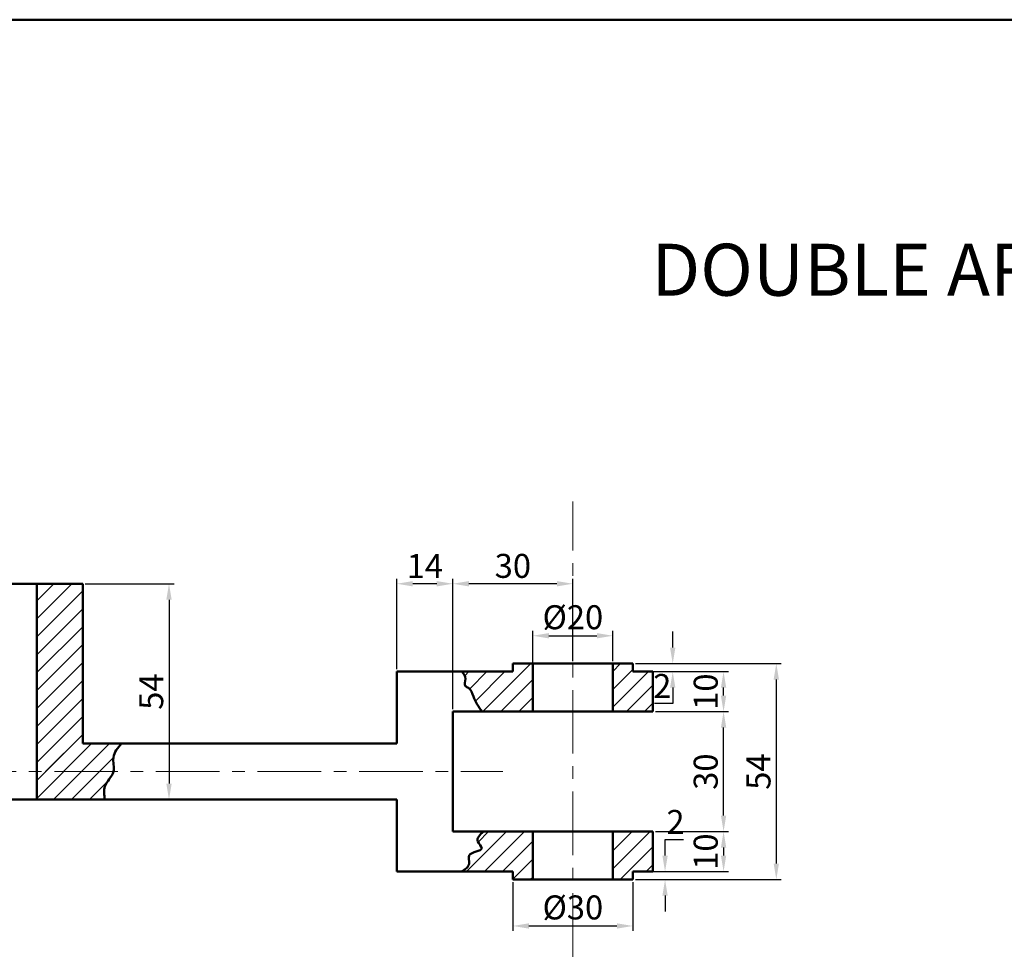
# Model space of a CAD drawing. Units: millimetres. Extents: x -1099 to -222, y 37 to 495.
# Tile 2 of 3: x -920 to -674, y 263 to 495. Entities that reach past the tile are written whole.
import ezdxf

# ---------------------------------------------------------------- set-up
doc = ezdxf.new("R2010")
doc.units = ezdxf.units.MM
doc.header["$LTSCALE"] = 0.5
doc.linetypes.add('CENTER', pattern=[50.800000000000004, 31.75, -6.349999999999999, 6.349999999999999, -6.349999999999999])
for name, color, linetype, lineweight in [('M-CNTR', 1, 'CENTER', 18), ('M-DIMS', 2, 'Continuous', 25), ('M-HATC', 8, 'Continuous', 18), ('M-OUTL', 7, 'Continuous', 50), ('M-TEXT', 7, 'Continuous', 25), ('M-TTLB', 7, 'Continuous', 50)]:
    doc.layers.add(name, color=color, linetype=linetype, lineweight=lineweight)
doc.styles.get("Standard").update_dxf_attribs({"font": 'arial.ttf'})
doc.dimstyles.new('ISO-25', dxfattribs={"dimtxt": 6, "dimasz": 4, "dimexe": 1.25, "dimexo": 0.625, "dimtad": 1, "dimtoh": 1, "dimtxsty": 'Standard', "dimcen": 2.5, "dimadec": 0, "dimazin": 0, "dimtfac": 1, "dimtofl": 0, "dimtmove": 0, "dimatfit": 3, "dimfxl": 1, "dimarcsym": 0})
pattern_1 = [(45, (-1406.913769851486, -374.9261606673909), (-2.245064030267288, 2.245064030267288), [])]

# ---------------------------------------------------------------- blocks, each defined once
blk = doc.blocks.new('*D8')
at = {"layer": 'Defpoints', "color": 0, "transparency": 16777216}
for p in [(-796.41964155178, 280.3451799427145), (-766.41964155178, 280.3451799427145), (-766.41964155178, 268.7543255228883)]:
    blk.add_point(p, dxfattribs=at)
at = {"layer": 'M-DIMS', "color": 0, "lineweight": -2, "transparency": 16777216}
for p, q in [((-796.41964155178, 279.7201799427145), (-796.41964155178, 267.5043255228883)), ((-766.41964155178, 279.7201799427145), (-766.41964155178, 267.5043255228883)), ((-792.41964155178, 268.7543255228883), (-770.41964155178, 268.7543255228883))]:
    blk.add_line(p, q, dxfattribs=at)
at = {"layer": 'M-DIMS', "color": 0, "transparency": 16777216}
for points in [[(-792.41964155178, 269.4209921895549), (-792.41964155178, 268.0876588562216), (-796.41964155178, 268.7543255228883)], [(-770.41964155178, 269.4209921895549), (-770.41964155178, 268.0876588562216), (-766.41964155178, 268.7543255228883)]]:
    blk.add_solid(points, dxfattribs=at)
at = {"layer": 'M-DIMS', "color": 0, "transparency": 16777216, "insert": (-781.41964155178, 272.6105669962853), "char_height": 6, "attachment_point": 5}
blk.add_mtext('%%C30', dxfattribs=at)
blk = doc.blocks.new('*D9')
at = {"layer": 'Defpoints', "color": 0, "transparency": 16777216}
for p in [(-761.4196415517803, 292.3451799427147), (-766.4196415517803, 282.3451799427146), (-743.7539602163725, 282.3451799427146)]:
    blk.add_point(p, dxfattribs=at)
at = {"layer": 'M-DIMS', "color": 0, "lineweight": -2, "transparency": 16777216}
for p, q in [((-760.7946415517802, 292.3451799427147), (-742.5039602163725, 292.3451799427147)), ((-743.7539602163725, 288.3451799427147), (-743.7539602163725, 286.3451799427146)), ((-765.7946415517804, 282.3451799427146), (-742.5039602163725, 282.3451799427146))]:
    blk.add_line(p, q, dxfattribs=at)
at = {"layer": 'M-DIMS', "color": 0, "transparency": 16777216}
for points in [[(-744.4206268830392, 288.3451799427147), (-743.0872935497059, 288.3451799427147), (-743.7539602163725, 292.3451799427147)], [(-744.4206268830392, 286.3451799427146), (-743.0872935497059, 286.3451799427146), (-743.7539602163725, 282.3451799427146)]]:
    blk.add_solid(points, dxfattribs=at)
at = {"layer": 'M-DIMS', "color": 0, "transparency": 16777216, "insert": (-747.4423981427024, 287.3451799427148), "char_height": 6, "attachment_point": 5, "rotation": 90}
blk.add_mtext('10', dxfattribs=at)
blk = doc.blocks.new('*D10')
at = {"layer": 'Defpoints', "color": 0, "transparency": 16777216}
for p in [(-761.4196415517803, 322.3451799427146), (-743.7539602163716, 322.3451799427146), (-761.4196415517803, 292.3451799427147)]:
    blk.add_point(p, dxfattribs=at)
at = {"layer": 'M-DIMS', "color": 0, "lineweight": -2, "transparency": 16777216}
for p, q in [((-760.7946415517802, 322.3451799427146), (-742.5039602163716, 322.3451799427146)), ((-743.7539602163716, 296.3451799427147), (-743.7539602163716, 318.3451799427146)), ((-760.7946415517802, 292.3451799427147), (-742.5039602163716, 292.3451799427147))]:
    blk.add_line(p, q, dxfattribs=at)
at = {"layer": 'M-DIMS', "color": 0, "transparency": 16777216}
for points in [[(-744.4206268830383, 318.3451799427146), (-743.087293549705, 318.3451799427146), (-743.7539602163716, 322.3451799427146)], [(-744.4206268830383, 296.3451799427147), (-743.087293549705, 296.3451799427147), (-743.7539602163716, 292.3451799427147)]]:
    blk.add_solid(points, dxfattribs=at)
at = {"layer": 'M-DIMS', "color": 0, "transparency": 16777216, "insert": (-747.4444445274218, 307.3451799427145), "char_height": 6, "attachment_point": 5, "rotation": 90}
blk.add_mtext('30', dxfattribs=at)
blk = doc.blocks.new('*D11')
at = {"layer": 'Defpoints', "color": 0, "transparency": 16777216}
for p in [(-771.41964155178, 341.3193151238818), (-791.41964155178, 332.3451799427146), (-771.41964155178, 334.3451799427145)]:
    blk.add_point(p, dxfattribs=at)
at = {"layer": 'M-DIMS', "color": 0, "lineweight": -2, "transparency": 16777216}
for p, q in [((-791.41964155178, 332.9701799427146), (-791.41964155178, 342.5693151238818)), ((-771.41964155178, 334.9701799427145), (-771.41964155178, 342.5693151238818)), ((-787.41964155178, 341.3193151238818), (-775.41964155178, 341.3193151238818))]:
    blk.add_line(p, q, dxfattribs=at)
at = {"layer": 'M-DIMS', "color": 0, "transparency": 16777216}
for points in [[(-787.41964155178, 341.9859817905485), (-787.41964155178, 340.6526484572152), (-791.41964155178, 341.3193151238818)], [(-775.41964155178, 341.9859817905485), (-775.41964155178, 340.6526484572152), (-771.41964155178, 341.3193151238818)]]:
    blk.add_solid(points, dxfattribs=at)
at = {"layer": 'M-DIMS', "color": 0, "transparency": 16777216, "insert": (-781.41964155178, 345.1755565972788), "char_height": 6, "attachment_point": 5}
blk.add_mtext('%%C20', dxfattribs=at)
blk = doc.blocks.new('*D12')
at = {"layer": 'Defpoints', "color": 0, "transparency": 16777216}
for p in [(-811.41964155178, 354.3253229173946), (-781.41964155178, 334.3451799427146), (-811.41964155178, 322.3451799427145)]:
    blk.add_point(p, dxfattribs=at)
at = {"layer": 'M-DIMS', "color": 0, "lineweight": -2, "transparency": 16777216}
for p, q in [((-811.41964155178, 322.9701799427145), (-811.41964155178, 355.5753229173946)), ((-781.41964155178, 334.9701799427146), (-781.41964155178, 355.5753229173946)), ((-785.41964155178, 354.3253229173946), (-807.4196415517802, 354.3253229173946))]:
    blk.add_line(p, q, dxfattribs=at)
at = {"layer": 'M-DIMS', "color": 0, "transparency": 16777216}
for points in [[(-807.4196415517802, 354.9919895840613), (-807.4196415517802, 353.6586562507279), (-811.41964155178, 354.3253229173946)], [(-785.41964155178, 354.9919895840613), (-785.41964155178, 353.6586562507279), (-781.41964155178, 354.3253229173946)]]:
    blk.add_solid(points, dxfattribs=at)
at = {"layer": 'M-DIMS', "color": 0, "transparency": 16777216, "insert": (-796.41964155178, 358.0158072284451), "char_height": 6, "attachment_point": 5}
blk.add_mtext('30', dxfattribs=at)
blk = doc.blocks.new('*D13')
at = {"layer": 'Defpoints', "color": 0, "transparency": 16777216}
for p in [(-825.41964155178, 354.3253229173948), (-825.41964155178, 332.3451799427147), (-811.41964155178, 322.3451799427145)]:
    blk.add_point(p, dxfattribs=at)
at = {"layer": 'M-DIMS', "color": 0, "lineweight": -2, "transparency": 16777216}
for p, q in [((-825.41964155178, 332.9701799427147), (-825.41964155178, 355.5753229173948)), ((-811.41964155178, 322.9701799427145), (-811.41964155178, 355.5753229173948)), ((-815.4196415517802, 354.3253229173948), (-821.41964155178, 354.3253229173948))]:
    blk.add_line(p, q, dxfattribs=at)
at = {"layer": 'M-DIMS', "color": 0, "transparency": 16777216}
for points in [[(-821.41964155178, 354.9919895840615), (-821.41964155178, 353.6586562507281), (-825.41964155178, 354.3253229173948)], [(-815.4196415517802, 354.9919895840615), (-815.4196415517802, 353.6586562507281), (-811.41964155178, 354.3253229173948)]]:
    blk.add_solid(points, dxfattribs=at)
at = {"layer": 'M-DIMS', "color": 0, "transparency": 16777216, "insert": (-818.41964155178, 357.9626012257167), "char_height": 6, "attachment_point": 5}
blk.add_mtext('14', dxfattribs=at)
blk = doc.blocks.new('*D14')
at = {"layer": 'Defpoints', "color": 0, "transparency": 16777216}
for p in [(-766.4196415517803, 334.3451799427147), (-766.41964155178, 280.3451799427147), (-730.5763774681391, 280.3451799427147)]:
    blk.add_point(p, dxfattribs=at)
at = {"layer": 'M-DIMS', "color": 0, "lineweight": -2, "transparency": 16777216}
for p, q in [((-765.7946415517804, 334.3451799427147), (-729.3263774681392, 334.3451799427147)), ((-730.5763774681391, 330.3451799427147), (-730.5763774681391, 284.3451799427147)), ((-765.79464155178, 280.3451799427147), (-729.3263774681392, 280.3451799427147))]:
    blk.add_line(p, q, dxfattribs=at)
at = {"layer": 'M-DIMS', "color": 0, "transparency": 16777216}
for points in [[(-731.2430441348058, 330.3451799427147), (-729.9097108014726, 330.3451799427147), (-730.5763774681391, 334.3451799427147)], [(-731.2430441348058, 284.3451799427147), (-729.9097108014726, 284.3451799427147), (-730.5763774681391, 280.3451799427147)]]:
    blk.add_solid(points, dxfattribs=at)
at = {"layer": 'M-DIMS', "color": 0, "transparency": 16777216, "insert": (-734.2525370861472, 307.3451799427149), "char_height": 6, "attachment_point": 5, "rotation": 90}
blk.add_mtext('54', dxfattribs=at)
blk = doc.blocks.new('*D15')
at = {"layer": 'Defpoints', "color": 0, "transparency": 16777216}
for p in [(-761.4196415517803, 282.3451799427147), (-758.3850048108699, 282.3451799427147), (-766.4196415517803, 280.3451799427146)]:
    blk.add_point(p, dxfattribs=at)
at = {"layer": 'M-DIMS', "color": 0, "lineweight": -2, "transparency": 16777216}
for p, q in [((-758.3850048108699, 286.3451799427148), (-758.3850048108699, 290.3451799427148)), ((-758.3850048108699, 290.3451799427148), (-753.785925683994, 290.3451799427148)), ((-760.7946415517802, 282.3451799427147), (-757.1350048108699, 282.3451799427147)), ((-765.7946415517804, 280.3451799427146), (-757.1350048108699, 280.3451799427146)), ((-758.3850048108699, 276.3451799427146), (-758.3850048108699, 272.3451799427146))]:
    blk.add_line(p, q, dxfattribs=at)
at = {"layer": 'M-DIMS', "color": 0, "transparency": 16777216}
for points in [[(-759.0516714775365, 286.3451799427148), (-757.7183381442032, 286.3451799427148), (-758.3850048108699, 282.3451799427147)], [(-759.0516714775365, 276.3451799427146), (-757.7183381442032, 276.3451799427146), (-758.3850048108699, 280.3451799427146)]]:
    blk.add_solid(points, dxfattribs=at)
at = {"layer": 'M-DIMS', "color": 0, "transparency": 16777216, "insert": (-755.7729652474316, 293.9824582510369), "char_height": 6, "attachment_point": 5}
blk.add_mtext('2', dxfattribs=at)
blk = doc.blocks.new('*D16')
at = {"layer": 'Defpoints', "color": 0, "transparency": 16777216}
for p in [(-761.4196415517803, 332.3451799427147), (-743.753960216372, 332.3451799427147), (-761.4196415517803, 322.3451799427146)]:
    blk.add_point(p, dxfattribs=at)
at = {"layer": 'M-DIMS', "color": 0, "lineweight": -2, "transparency": 16777216}
for p, q in [((-760.7946415517804, 332.3451799427147), (-742.5039602163721, 332.3451799427147)), ((-743.753960216372, 326.3451799427147), (-743.753960216372, 328.3451799427147)), ((-760.7946415517802, 322.3451799427146), (-742.5039602163721, 322.3451799427146))]:
    blk.add_line(p, q, dxfattribs=at)
at = {"layer": 'M-DIMS', "color": 0, "transparency": 16777216}
for points in [[(-744.4206268830387, 328.3451799427147), (-743.0872935497054, 328.3451799427147), (-743.753960216372, 332.3451799427147)], [(-744.4206268830387, 326.3451799427147), (-743.0872935497054, 326.3451799427147), (-743.753960216372, 322.3451799427146)]]:
    blk.add_solid(points, dxfattribs=at)
at = {"layer": 'M-DIMS', "color": 0, "transparency": 16777216, "insert": (-747.442398142702, 327.3451799427148), "char_height": 6, "attachment_point": 5, "rotation": 90}
blk.add_mtext('10', dxfattribs=at)
blk = doc.blocks.new('*D17')
at = {"layer": 'Defpoints', "color": 0, "transparency": 16777216}
for p in [(-766.4196415517803, 334.3451799427147), (-766.4196415517803, 332.3451799427147), (-756.4613537627584, 332.3451799427147)]:
    blk.add_point(p, dxfattribs=at)
at = {"layer": 'M-DIMS', "color": 0, "lineweight": -2, "transparency": 16777216}
for p, q in [((-756.4613537627584, 338.3451799427147), (-756.4613537627584, 342.3451799427147)), ((-765.7946415517804, 334.3451799427147), (-755.2113537627584, 334.3451799427147)), ((-765.7946415517804, 332.3451799427147), (-755.2113537627584, 332.3451799427147)), ((-756.4613537627584, 328.3451799427147), (-756.4613537627584, 324.3451799427147)), ((-756.4613537627584, 324.3451799427147), (-761.0604328896343, 324.3451799427147))]:
    blk.add_line(p, q, dxfattribs=at)
at = {"layer": 'M-DIMS', "color": 0, "transparency": 16777216}
for points in [[(-757.128020429425, 338.3451799427147), (-755.7946870960918, 338.3451799427147), (-756.4613537627584, 334.3451799427147)], [(-757.128020429425, 328.3451799427147), (-755.7946870960918, 328.3451799427147), (-756.4613537627584, 332.3451799427147)]]:
    blk.add_solid(points, dxfattribs=at)
at = {"layer": 'M-DIMS', "color": 0, "transparency": 16777216, "insert": (-759.0733933261962, 327.9824582510368), "char_height": 6, "attachment_point": 5}
blk.add_mtext('2', dxfattribs=at)
blk = doc.blocks.new('*D18')
at = {"layer": 'Defpoints', "color": 0, "transparency": 16777216}
for p in [(-903.9196415517805, 354.3451799427146), (-903.9196415517805, 300.3451799427147), (-882.3550305426962, 300.3451799427147)]:
    blk.add_point(p, dxfattribs=at)
at = {"layer": 'M-DIMS', "color": 0, "lineweight": -2, "transparency": 16777216}
for p, q in [((-903.2946415517805, 354.3451799427146), (-881.1050305426963, 354.3451799427147)), ((-882.3550305426962, 350.3451799427147), (-882.3550305426962, 304.3451799427147)), ((-903.2946415517805, 300.3451799427147), (-881.1050305426963, 300.3451799427147))]:
    blk.add_line(p, q, dxfattribs=at)
at = {"layer": 'M-DIMS', "color": 0, "transparency": 16777216}
for points in [[(-883.021697209363, 350.3451799427147), (-881.6883638760296, 350.3451799427147), (-882.3550305426962, 354.3451799427147)], [(-883.021697209363, 304.3451799427147), (-881.6883638760296, 304.3451799427147), (-882.3550305426962, 300.3451799427147)]]:
    blk.add_solid(points, dxfattribs=at)
at = {"layer": 'M-DIMS', "color": 0, "transparency": 16777216, "insert": (-886.0311901607042, 327.3451799427149), "char_height": 6, "attachment_point": 5, "rotation": 90}
blk.add_mtext('54', dxfattribs=at)

msp = doc.modelspace()

# ---------------------------------------------------------------- hatches: boundary and pattern name
at = {"layer": 'M-HATC', "ltscale": 0.5}
h = msp.add_hatch(dxfattribs=at)
h.set_pattern_fill('ANSI31', color=256)
h.set_pattern_definition(pattern_1)
edge = h.paths.add_edge_path()
edge.add_line((-523.0471990713963, 354.3451799427145), (-536.5471990713963, 354.3451799427145))
edge.add_line((-536.5471990713963, 354.3451799427145), (-536.5471990713962, 314.3451799427146))
edge.add_line((-536.5471990713962, 314.3451799427146), (-552.3843475483716, 314.3451799427146))
edge.add_spline(control_points=[(-552.3843475483715, 314.3451799427146), (-549.8505565574773, 313.6991421584863), (-544.7780436710062, 312.4058093629157), (-548.7645988707294, 305.0728376077207), (-543.3062567676095, 303.3599159072043), (-542.293612313991, 300.4754585651784), (-541.5457368643287, 298.3451799427145)], knot_values=[0, 0, 0, 0, 6.339962572469942, 12.69226308096105, 14.93837176657165, 21.28280604000792, 21.28280604000792, 21.28280604000792, 21.28280604000792], degree=3, periodic=0)
edge.add_line((-541.5457368643287, 298.3451799427145), (-536.5471990713962, 298.3451799427145))
edge.add_line((-536.5471990713962, 298.3451799427145), (-536.5471990713962, 289.3451799427145))
edge.add_line((-536.5471990713962, 289.3451799427145), (-523.0471990713963, 289.3451799427145))
edge.add_line((-523.0471990713963, 289.3451799427145), (-523.0471990713963, 354.3451799427145))
edge = h.paths.add_edge_path()
edge.add_spline(control_points=[(-455.5050825523017, 298.3451799427145), (-454.6057138850319, 301.2161322334999), (-453.229947160803, 305.6078358498839), (-460.3887949936558, 306.6902340845678), (-457.2427831204656, 312.8516918255611), (-460.860805180341, 313.8622299753194), (-462.5899072793266, 314.3451799427146)], knot_values=[0, 0, 0, 0, 7.055104645909409, 10.79221298342518, 15.64668287420668, 20.09042546330913, 20.09042546330913, 20.09042546330913, 20.09042546330913], degree=3, periodic=0)
edge.add_line((-462.5899072793263, 314.3451799427145), (-471.5471990713964, 314.3451799427145))
edge.add_line((-471.5471990713964, 314.3451799427145), (-471.5471990713963, 354.3451799427145))
edge.add_line((-471.5471990713963, 354.3451799427145), (-485.0471990713963, 354.3451799427145))
edge.add_line((-485.0471990713963, 354.3451799427145), (-485.0471990713963, 289.3451799427145))
edge.add_line((-485.0471990713963, 289.3451799427145), (-471.5471990713964, 289.3451799427145))
edge.add_line((-471.5471990713964, 289.3451799427145), (-471.5471990713964, 298.3451799427145))
edge.add_line((-471.5471990713964, 298.3451799427145), (-455.5050825523017, 298.3451799427145))
edge = h.paths.add_edge_path()
edge.add_line((-903.91964155178, 354.3451799427145), (-915.4196415517802, 354.3451799427145))
edge.add_line((-915.4196415517802, 354.3451799427145), (-915.4196415517802, 307.3451799427145))
edge.add_line((-915.4196415517802, 307.3451799427145), (-896.253112336959, 307.3451799427145))
edge.add_spline(control_points=[(-896.2531123369574, 307.3451799427255), (-895.980146866338, 308.4515450050575), (-896.887919395419, 311.2066129734494), (-895.167283921143, 313.2574011399624), (-894.2546246681089, 314.3451799427146)], knot_values=[0, 1.16289e-11, 1.16289e-11, 1.16289e-11, 3.538517819249876, 7.535493156952304, 7.535493156952304, 7.535493156952304, 7.535493156952304], degree=3, periodic=0)
edge.add_line((-894.2546246681089, 314.3451799427146), (-903.91964155178, 314.3451799427146))
edge.add_line((-903.91964155178, 314.3451799427146), (-903.91964155178, 354.3451799427145))
edge = h.paths.add_edge_path()
edge.add_spline(control_points=[(-898.3868935517232, 300.3451799427145), (-898.5643230712737, 301.4941162137897), (-898.970914129592, 304.1269769439559), (-896.582317175395, 306.0108693034795), (-896.2531123369583, 307.3451799427219)], knot_values=[7.535493156940674, 7.535493156940674, 7.535493156940674, 7.535493156940674, 10.83967568073524, 15.10723811026111, 15.10723811027274, 15.10723811027274, 15.10723811027274], degree=3, periodic=0)
edge.add_line((-896.25311233696, 307.3451799427145), (-915.4196415517802, 307.3451799427145))
edge.add_line((-915.4196415517802, 307.3451799427145), (-915.4196415517802, 300.3451799427145))
edge.add_line((-915.4196415517802, 300.3451799427145), (-898.3868935517232, 300.3451799427145))
h = msp.add_hatch(dxfattribs=at)
h.set_pattern_fill('ANSI31', color=256)
h.set_pattern_definition(pattern_1)
edge = h.paths.add_edge_path()
edge.add_line((-791.41964155178, 292.3451799427145), (-803.788806237629, 292.3451799427145))
edge.add_spline(control_points=[(-803.788806237629, 292.3451799427145), (-804.6430356722922, 291.5636625158688), (-806.0957601286138, 290.2345939624444), (-802.7883338705159, 287.4254447496014), (-808.2615396944161, 287.3348708991068), (-806.7701582095196, 283.880750434352), (-808.3541580520874, 282.9118064617069), (-809.2804616797661, 282.3451799427145)], knot_values=[0, 0, 0, 0, 2.816293269149902, 4.789460468405914, 8.397554328858256, 10.40129909934276, 13.22338626941326, 13.22338626941326, 13.22338626941326, 13.22338626941326], degree=3, periodic=0)
edge.add_line((-809.2804616797661, 282.3451799427145), (-796.41964155178, 282.3451799427145))
edge.add_line((-796.41964155178, 282.3451799427145), (-796.41964155178, 280.3451799427145))
edge.add_line((-796.41964155178, 280.3451799427145), (-791.41964155178, 280.3451799427145))
edge.add_line((-791.41964155178, 280.3451799427145), (-791.41964155178, 292.3451799427145))
h.paths.add_polyline_path([(-761.4196415517802, 292.3451799427145), (-771.41964155178, 292.3451799427145), (-771.41964155178, 280.3451799427146), (-766.41964155178, 280.3451799427146), (-766.41964155178, 282.3451799427146), (-761.4196415517802, 282.3451799427146)])
h.paths.add_polyline_path([(-761.4196415517802, 332.3451799427145), (-766.41964155178, 332.3451799427145), (-766.41964155178, 334.3451799427145), (-771.41964155178, 334.3451799427145), (-771.41964155178, 322.3451799427146), (-761.4196415517802, 322.3451799427146)])
edge = h.paths.add_edge_path()
edge.add_line((-791.41964155178, 334.3451799427146), (-796.41964155178, 334.3451799427146))
edge.add_line((-796.41964155178, 334.3451799427146), (-796.41964155178, 332.3451799427146))
edge.add_line((-796.41964155178, 332.3451799427146), (-825.41964155178, 332.3451799427147))
edge.add_line((-825.41964155178, 332.3451799427147), (-825.41964155178, 314.3451799427146))
edge.add_line((-825.41964155178, 314.3451799427146), (-894.2546246681089, 314.3451799427146))
edge.add_spline(control_points=[(-894.2546246681089, 314.3451799427146), (-895.167283921143, 313.2574011399624), (-896.887919395419, 311.2066129734494), (-895.980146866338, 308.4515450050575), (-896.2531123369574, 307.3451799427255)], knot_values=[0, 0, 0, 0, 3.996975337702428, 7.535493156940675, 7.535493156940675, 7.535493156940675, 7.535493156952304], degree=3, periodic=0)
edge.add_line((-896.2531123369592, 307.3451799427145), (-811.41964155178, 307.3451799427145))
edge.add_line((-811.41964155178, 307.3451799427145), (-811.41964155178, 322.3451799427145))
edge.add_line((-811.41964155178, 322.3451799427145), (-791.41964155178, 322.3451799427145))
edge.add_line((-791.41964155178, 322.3451799427145), (-791.41964155178, 334.3451799427146))
edge = h.paths.add_edge_path(flags=17)
edge.add_line((-791.41964155178, 334.3451799427146), (-796.41964155178, 334.3451799427146))
edge.add_line((-796.41964155178, 334.3451799427146), (-796.41964155178, 332.3451799427146))
edge.add_line((-796.41964155178, 332.3451799427146), (-809.1458764513367, 332.3451799427146))
edge.add_spline(control_points=[(-809.1458764513367, 332.3451799427146), (-808.7045923475155, 331.8016482585959), (-807.8604577341806, 330.7619237273116), (-808.7787640513174, 328.7415445402653), (-806.8533195247304, 328.1609172035829), (-806.2334382476537, 325.3667754924555), (-804.9288864716057, 323.519937991929), (-804.099071883645, 322.3451799427145)], knot_values=[0, 0, 0, 0, 2.00655280180981, 3.838345090666528, 4.674747458122268, 7.17505285740918, 11.54544967221059, 11.54544967221059, 11.54544967221059, 11.54544967221059], degree=3, periodic=0)
edge.add_line((-804.099071883645, 322.3451799427145), (-791.41964155178, 322.3451799427145))
edge.add_line((-791.41964155178, 322.3451799427145), (-791.41964155178, 334.3451799427146))
h.paths.add_polyline_path([(-791.41964155178, 334.3451799427146), (-796.41964155178, 334.3451799427146), (-796.41964155178, 332.3451799427146), (-809.1458764513367, 332.3451799427146), (-825.41964155178, 332.3451799427147), (-825.41964155178, 314.3451799427146), (-894.2546246681089, 314.3451799427146), (-903.91964155178, 314.3451799427146), (-903.91964155178, 354.3451799427145), (-915.4196415517802, 354.3451799427146), (-915.4196415517802, 307.3451799427145), (-811.41964155178, 307.3451799427145), (-811.41964155178, 322.3451799427145), (-791.41964155178, 322.3451799427145)])

# ---------------------------------------------------------------- linework, layer by layer
at = {"layer": 'M-CNTR'}
for p, q in [((-781.41964155178, 134.0656101931836), (-781.41964155178, 374.8729414708104)), ((-1088.8088415032, 307.3451799427145), (-798.9646638206668, 307.3451799427145))]:
    msp.add_line(p, q, dxfattribs=at)
at = {"layer": 'M-OUTL'}
for p, q in [((-968.9196415517802, 354.3451799427145), (-903.91964155178, 354.3451799427145)), ((-915.4196415517802, 300.3451799427145), (-915.4196415517802, 354.3451799427145)), ((-903.91964155178, 314.3451799427146), (-903.91964155178, 354.3451799427145)), ((-825.41964155178, 332.3451799427147), (-825.41964155178, 314.3451799427146)), ((-796.41964155178, 332.3451799427146), (-825.41964155178, 332.3451799427147)), ((-766.41964155178, 334.3451799427145), (-796.41964155178, 334.3451799427146)), ((-796.41964155178, 334.3451799427145), (-796.41964155178, 332.3451799427146)), ((-791.41964155178, 334.3451799427145), (-791.41964155178, 322.3451799427146)), ((-771.41964155178, 334.3451799427145), (-771.41964155178, 322.3451799427146)), ((-766.41964155178, 334.3451799427145), (-766.41964155178, 332.3451799427145)), ((-761.41964155178, 332.3451799427145), (-766.41964155178, 332.3451799427145)), ((-761.4196415517802, 332.3451799427145), (-761.4196415517802, 322.3451799427146)), ((-761.41964155178, 322.3451799427146), (-811.41964155178, 322.3451799427145)), ((-811.41964155178, 322.3451799427145), (-811.41964155178, 292.3451799427145)), ((-903.91964155178, 314.3451799427146), (-825.41964155178, 314.3451799427146)), ((-1063.41964155178, 300.3451799427145), (-825.41964155178, 300.3451799427145)), ((-825.41964155178, 300.3451799427145), (-825.41964155178, 282.3451799427145)), ((-761.41964155178, 292.3451799427145), (-811.41964155178, 292.3451799427145)), ((-791.41964155178, 292.3451799427145), (-791.41964155178, 280.3451799427145)), ((-771.41964155178, 292.3451799427145), (-771.41964155178, 280.3451799427145)), ((-761.4196415517802, 292.3451799427145), (-761.4196415517802, 282.3451799427147)), ((-796.4196415517802, 282.3451799427145), (-825.41964155178, 282.3451799427145)), ((-796.41964155178, 282.3451799427145), (-796.41964155178, 280.3451799427145)), ((-761.41964155178, 282.3451799427147), (-766.41964155178, 282.3451799427147)), ((-761.4196415517802, 282.3451799427146), (-766.41964155178, 282.3451799427146)), ((-766.41964155178, 282.3451799427145), (-766.41964155178, 280.3451799427145)), ((-766.41964155178, 280.3451799427146), (-796.41964155178, 280.3451799427145))]:
    msp.add_line(p, q, dxfattribs=at)
for points, knots in [([(-804.099071883645, 322.3451799427145), (-804.9288864716059, 323.5199379919291), (-806.233438247654, 325.3667754924557), (-806.8533195247304, 328.160917203583), (-808.7787640513174, 328.7415445402652), (-807.8604577341803, 330.7619237273116), (-808.7045923475155, 331.8016482585959), (-809.1458764513367, 332.3451799427146)], [0, 0, 0, 0, 4.370396814801415, 6.870702214088328, 7.707104581544068, 9.538896870400787, 11.5454496722106, 11.5454496722106, 11.5454496722106, 11.5454496722106]), ([(-894.2546246681089, 314.3451799427146), (-895.167283921143, 313.2574011399624), (-896.8879193954219, 311.2066129734463), (-895.4660496653961, 306.8912722653842), (-898.970914129592, 304.126976943956), (-898.5643230712735, 301.4941162137897), (-898.3868935517232, 300.3451799427145)], [0, 0, 0, 0, 3.996975337702428, 7.535493156952304, 11.80305558647818, 15.10723811027274, 15.10723811027274, 15.10723811027274, 15.10723811027274]), ([(-803.788806237629, 292.3451799427145), (-804.6430356722922, 291.5636625158688), (-806.0957601286138, 290.2345939624444), (-802.7883338705159, 287.4254447496014), (-808.2615396944161, 287.3348708991068), (-806.7701582095196, 283.880750434352), (-808.3541580520874, 282.9118064617069), (-809.2804616797661, 282.3451799427145)], [0, 0, 0, 0, 2.816293269149902, 4.789460468405914, 8.397554328858256, 10.40129909934276, 13.22338626941326, 13.22338626941326, 13.22338626941326, 13.22338626941326])]:
    msp.add_open_spline(points, degree=3, knots=knots, dxfattribs=at)
at = {"layer": 'M-TTLB', "ltscale": 0.5}
msp.add_lwpolyline([(-1099.004687419986, 495.3704252679146), (-222.2054647419409, 495.3704252679146), (-222.2054647419409, 36.58144759589982), (-1099.004687419986, 36.58144759589982)], close=True, dxfattribs=at)

# ---------------------------------------------------------------- texts
at = {"layer": 'M-TEXT', "ltscale": 0.5, "insert": (-761.7915721372545, 439.3437857891166), "char_height": 13, "attachment_point": 1}
msp.add_mtext_dynamic_manual_height_columns('DOUBLE ARM LEVER', width=201.8957420871643, gutter_width=12.5, heights=[0], dxfattribs=at)

# ---------------------------------------------------------------- dimensions: what is measured, and where the dimension line sits
at = {"layer": 'M-DIMS'}
for base, p1, p2, picture, middle in [((-825.41964155178, 354.3253229173948), (-811.41964155178, 322.3451799427145), (-825.41964155178, 332.3451799427147), '*D13', (-818.41964155178, 357.9626012257167)), ((-811.41964155178, 354.3253229173946), (-781.41964155178, 334.3451799427146), (-811.41964155178, 322.3451799427145), '*D12', (-796.41964155178, 358.0158072284451))]:
    dim = msp.add_linear_dim(base=base, p1=p1, p2=p2, dimstyle='ISO-25', override={"dimclrd": 0, "dimclre": 0, "dimclrt": 0}, dxfattribs=at)
    dim.commit()
    dim.dimension.update_dxf_attribs({"geometry": picture, "text_midpoint": middle})
for base, p1, p2, picture, middle in [((-882.3550305426962, 300.3451799427147), (-903.91964155178, 354.3451799427145), (-903.91964155178, 300.3451799427145), '*D18', (-886.0311901607042, 327.3451799427149)), ((-756.4613537627584, 332.3451799427147), (-766.41964155178, 334.3451799427145), (-766.41964155178, 332.3451799427145), '*D17', (-759.0733933261962, 327.9824582510368)), ((-730.5763774681391, 280.3451799427147), (-766.41964155178, 334.3451799427145), (-766.4196415517799, 280.3451799427146), '*D14', (-734.2525370861472, 307.3451799427149)), ((-743.753960216372, 332.3451799427147), (-761.41964155178, 322.3451799427146), (-761.4196415517802, 332.3451799427145), '*D16', (-747.442398142702, 327.3451799427148)), ((-758.3850048108699, 282.3451799427147), (-766.41964155178, 280.3451799427145), (-761.41964155178, 282.3451799427147), '*D15', (-755.7729652474316, 293.9824582510369)), ((-743.7539602163725, 282.3451799427146), (-761.41964155178, 292.3451799427145), (-766.41964155178, 282.3451799427145), '*D9', (-747.4423981427024, 287.3451799427148))]:
    dim = msp.add_linear_dim(base=base, p1=p1, p2=p2, angle=90, dimstyle='ISO-25', override={"dimclrd": 0, "dimclre": 0, "dimclrt": 0}, dxfattribs=at)
    dim.commit()
    dim.dimension.update_dxf_attribs({"geometry": picture, "text_midpoint": middle})
for base, p1, p2, picture, middle in [((-771.41964155178, 341.3193151238818), (-791.41964155178, 332.3451799427146), (-771.41964155178, 334.3451799427145), '*D11', (-781.41964155178, 345.1755565972788)), ((-766.41964155178, 268.7543255228883), (-796.41964155178, 280.3451799427145), (-766.41964155178, 280.3451799427145), '*D8', (-781.41964155178, 272.6105669962853))]:
    dim = msp.add_linear_dim(base=base, p1=p1, p2=p2, text='%%C<>', dimstyle='ISO-25', override={"dimclrd": 0, "dimclre": 0, "dimclrt": 0}, dxfattribs=at)
    dim.commit()
    dim.dimension.update_dxf_attribs({"geometry": picture, "text_midpoint": middle})
dim = msp.add_linear_dim(base=(-743.7539602163716, 322.3451799427146), p1=(-761.41964155178, 292.3451799427145), p2=(-761.41964155178, 322.3451799427146), angle=90, dimstyle='ISO-25', override={"dimclrd": 0, "dimclre": 0, "dimclrt": 0}, dxfattribs=at)
dim.commit()
dim.dimension.update_dxf_attribs({"geometry": '*D10', "text_midpoint": (-743.7539602163714, 307.3451799427145), "dimtype": 160})

doc.saveas('drawing.dxf')
